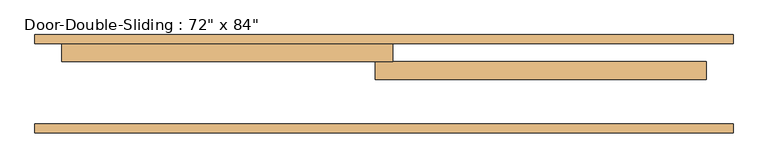
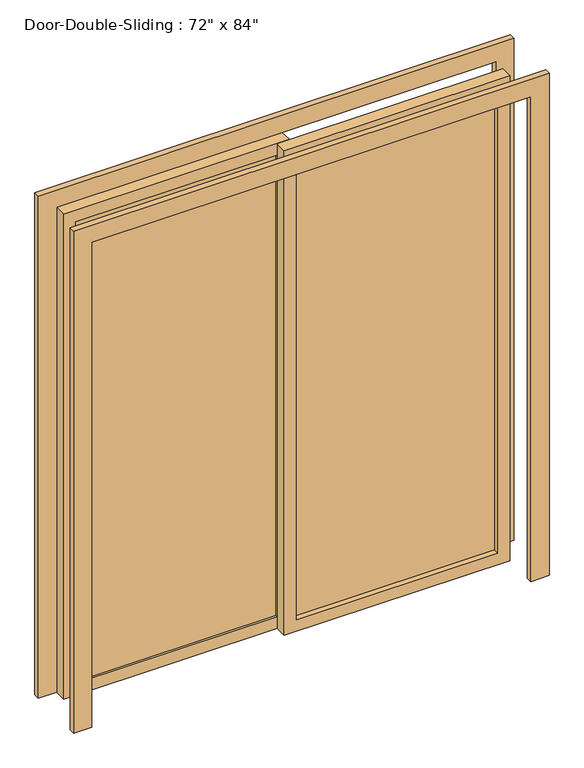
"""IFC4 building model written with IfcOpenShell, lengths in millimetres: door geometry."""

from ifc_helpers import new_model, si_unit, frame, origin, place, context, project, spatial, polyline, outline, extrude, source, transform, mapped, element, save


def door_d4d75d1e(model_context):
    return source(origin(), model_context, "Body", "SweptSolid", [
        extrude(outline(polyline([(0.0, 990.6), (2209.8, 990.6), (2209.8, -990.6), (0.0, -990.6), (0.0, -914.4), (2133.6, -914.4), (2133.6, 914.4), (0.0, 914.4), (0.0, 990.6)])), frame((0.0, 241.3, 0.0), z_axis=(0.0, 1.0, 0.0), x_axis=(0.0, 0.0, 1.0)), (0.0, 0.0, 1.0), 25.4),
        extrude(outline(polyline([(0.0, -990.6), (0.0, -914.4), (2133.6, -914.4), (2133.6, 914.4), (0.0, 914.4), (0.0, 990.6), (2209.8, 990.6), (2209.8, -990.6), (0.0, -990.6)])), frame((0.0, -12.7, 0.0), z_axis=(0.0, 1.0, 0.0), x_axis=(0.0, 0.0, 1.0)), (0.0, 0.0, 1.0), 25.4),
        extrude(outline(polyline([(2133.6, 25.4), (2133.6, -914.4), (0.0, -914.4), (0.0, 25.4), (2133.6, 25.4)]), holes=[polyline([(2082.8, -25.4), (50.8, -25.4), (50.8, -863.6), (2082.8, -863.6), (2082.8, -25.4)])]), frame((0.0, 190.5, 0.0), z_axis=(0.0, 1.0, 0.0), x_axis=(0.0, 0.0, 1.0)), (0.0, 0.0, 1.0), 50.8),
        extrude(outline(polyline([(2133.6, -25.4), (0.0, -25.4), (0.0, 914.4), (2133.6, 914.4), (2133.6, -25.4)]), holes=[polyline([(2082.8, 25.4), (2082.8, 863.6), (50.8, 863.6), (50.8, 25.4), (2082.8, 25.4)])]), frame((0.0, 139.7, 0.0), z_axis=(0.0, 1.0, 0.0), x_axis=(0.0, 0.0, 1.0)), (0.0, 0.0, 1.0), 50.8),
        extrude(outline(polyline([(-25.4, 200.025), (-863.6, 200.025), (-863.6, 206.375), (-25.4, 206.375), (-25.4, 200.025)])), frame((0.0, 0.0, 50.8), z_axis=(0.0, 0.0, 1.0), x_axis=(1.0, 0.0, 0.0)), (0.0, 0.0, 1.0), 2032.0),
        extrude(outline(polyline([(25.4, 168.275), (863.6, 168.275), (863.6, 161.925), (25.4, 161.925), (25.4, 168.275)])), frame((0.0, 0.0, 50.8), z_axis=(0.0, 0.0, 1.0), x_axis=(1.0, 0.0, 0.0)), (0.0, 0.0, 1.0), 2032.0),
    ])


if __name__ == "__main__":
    model = new_model("IFC4")
    model_context = context("Model", 3, world=origin())
    ifc_project = project(units=[si_unit("LENGTHUNIT", "METRE", prefix="MILLI")], contexts=[model_context])
    site = spatial("IfcSite", under=ifc_project)
    building = spatial("IfcBuilding", under=site)
    placement = place(None, origin())
    door_shape = door_d4d75d1e(model_context)
    element("IfcDoor", 1, ObjectType="Door-Double-Sliding : 72\" x 84\"", at=placement, inside=building, context=model_context, shape_type="MappedRepresentation", body=[
        mapped(door_shape, transform((0.0, 0.0, 0.0), x_axis=(1.0, 0.0, 0.0), y_axis=(0.0, 1.0, 0.0), z_axis=(0.0, 0.0, 1.0))),
    ])
    save(model, "model.ifc")

# Revit data of these elements
# Type "Door-Double-Sliding : 72\" x 84\""
#   Type Mark = "9"
#   Construction Type Id = "opn-d45"
#   Assembly Code = "C1020"
#   Analytic Construction = "Wood frame, double glass door "
#   Thickness = 0' - 2"
#   Thermal Resistance (R) = 1.8150 (h·ft²·°F)/BTU
#   Heat Transfer Coefficient (U) = 0.5510 BTU/(h·ft²·°F)
#   Height = 7' - 0"
#   Rail Width = 0' - 2"
#   Stiles = 0' - 2"
#   Trim Projection Ext = 0' - 1"
#   Trim Projection Int = 0' - 1"
#   Trim Width = 0' - 3"
#   Width = 6' - 0"
#   Define Thermal Properties by = 1
#   Glazing = Glass
#   Panel Material = Wood - Birch - Solid Stained Light Low Gloss
#   Trim Material = Paint - Sienna
#   Visual Light Transmittance = 0
#   Solar Heat Gain Coefficient = 0
#   Function = (empty or 0)
#   Wall Closure = (empty or 0)
# Element 1 (IfcDoor, "Door-Double-Sliding : 72\" x 84\"")
#   Materials on its faces: "Paint - Sienna", "Wood - Birch - Solid Stained Light Low Gloss", "Glass"
# Materials
#   "Glass": class "Glass", colour RGB 0 128 192, transparency 0.75, Description = "Soda Lime Glass", Cost = 0
#   "Wood - Birch - Solid Stained Light Low Gloss": class "Wood", colour RGB 210 159 95, transparency 0, Cost = 0
#   "Paint - Sienna": colour RGB 118 70 51, transparency 0, Cost = 0
